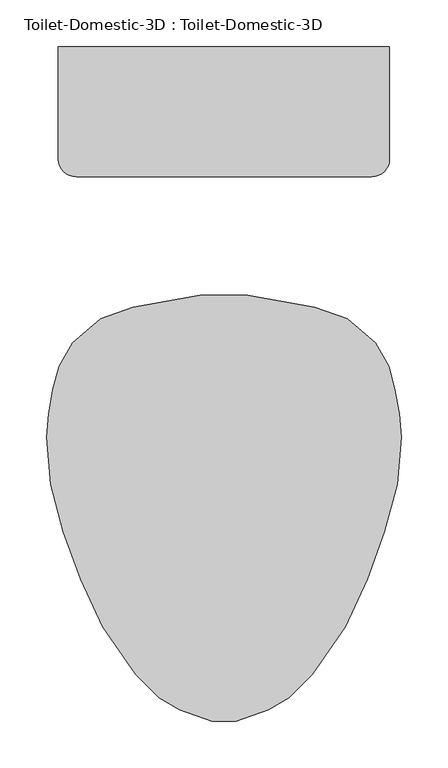
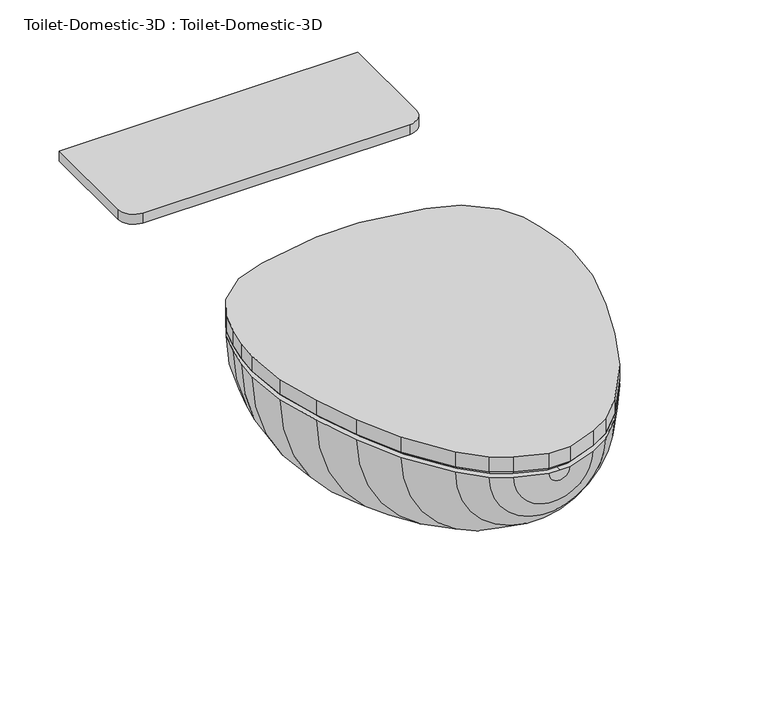
"""IFC4 building model written with IfcOpenShell, lengths in millimetres: flow terminal geometry, Toilet-Domestic-3D : Toilet-Domestic-3D."""

from ifc_helpers import new_model, si_unit, point, frame, frame_2d, origin, place, context, project, spatial, polyline, circle_curve, trimmed, segment, composite_curve, outline, extrude, faceted_brep, source, transform, mapped, element, save
from ifc_brep_helpers import plane_surface, revolved_surface, advanced_brep


def toilet_domestic_3d_toilet_domestic_3d_183bbd19(model_context):
    return source(origin(), model_context, "Body", "SolidModel", [
        advanced_brep(
        [(-25.4, 152.4, 361.95), (-97.4252791, 139.7, 361.95), (-132.3182423, 127.0, 361.95), (-162.5887836, 101.6, 361.95), (-176.9845865, 76.2, 361.95), (-183.790496, 50.8, 361.95), (-188.2862441, 25.3033453, 361.95), (-190.5, 0.0, 361.95), (-186.0724883, -50.6066907, 361.95), (-172.4088722, -101.6, 361.95), (-153.9191843, -152.4, 361.95), (-130.2307553, -203.2, 361.95), (-94.9900085, -254.0, 361.95), (-69.5900085, -279.4, 361.95), (-47.5929632, -292.1, 361.95), (-12.7, -304.8, 361.95), (0.0, -304.8, 361.95), (0.0, -284.592034, 361.95), (-12.5224565, -284.592034, 361.95), (-39.5113323, -274.7688865, 361.95), (-58.4178985, -263.8531754, 361.95), (-79.2146703, -243.0564036, 361.95), (-114.0255101, -192.8761202, 361.95), (-136.654021, -144.3491221, 361.95), (-154.575847, -95.1093097, 361.95), (-167.7238545, -46.0402777, 361.95), (-171.5645445, -2.1409906, 361.95), (-169.3087351, 23.6430284, 361.95), (-165.101298, 47.5045901, 361.95), (-159.5484355, 68.2281551, 361.95), (-146.1085923, 90.5605136, 361.95), (-121.9980886, 110.7916284, 361.95), (-94.1172813, 120.9394123, 361.95), (-22.0920022, 133.6394123, 361.95), (0.0, 133.6394123, 361.95), (0.0, 152.4, 361.95), (25.4, 152.4, 361.95), (22.0920022, 133.6394123, 361.95), (94.1172813, 120.9394123, 361.95), (121.9980886, 110.7916284, 361.95), (146.1085923, 90.5605136, 361.95), (159.5484355, 68.2281551, 361.95), (165.101298, 47.5045901, 361.95), (169.3087351, 23.6430284, 361.95), (171.5645445, -2.1409906, 361.95), (167.7238545, -46.0402777, 361.95), (154.575847, -95.1093097, 361.95), (136.654021, -144.3491221, 361.95), (114.0255101, -192.8761202, 361.95), (79.2146703, -243.0564036, 361.95), (58.4178985, -263.8531754, 361.95), (39.5113323, -274.7688865, 361.95), (12.5224565, -284.592034, 361.95), (12.7, -304.8, 361.95), (47.5929632, -292.1, 361.95), (69.5900085, -279.4, 361.95), (94.9900085, -254.0, 361.95), (130.2307553, -203.2, 361.95), (153.9191843, -152.4, 361.95), (172.4088722, -101.6, 361.95), (186.0724883, -50.6066907, 361.95), (190.5, 0.0, 361.95), (188.2862441, 25.3033453, 361.95), (183.790496, 50.8, 361.95), (176.9845865, 76.2, 361.95), (162.5887836, 101.6, 361.95), (132.3182423, 127.0, 361.95), (97.4252791, 139.7, 361.95)],
        [
            (0, 1),
            (1, 2),
            (2, 3),
            (3, 4),
            (4, 5),
            (5, 6),
            (6, 7),
            (7, 8),
            (8, 9),
            (9, 10),
            (10, 11),
            (11, 12),
            (12, 13),
            (13, 14),
            (14, 15),
            (15, 16),
            (16, 17),
            (17, 18),
            (18, 19),
            (19, 20),
            (20, 21),
            (21, 22),
            (22, 23),
            (23, 24),
            (24, 25),
            (25, 26),
            (26, 27),
            (27, 28),
            (28, 29),
            (29, 30),
            (30, 31),
            (31, 32),
            (32, 33),
            (33, 34),
            (34, 35),
            (35, 0),
            (36, 35),
            (34, 37),
            (37, 38),
            (38, 39),
            (39, 40),
            (40, 41),
            (41, 42),
            (42, 43),
            (43, 44),
            (44, 45),
            (45, 46),
            (46, 47),
            (47, 48),
            (48, 49),
            (49, 50),
            (50, 51),
            (51, 52),
            (52, 17),
            (16, 53),
            (53, 54),
            (54, 55),
            (55, 56),
            (56, 57),
            (57, 58),
            (58, 59),
            (59, 60),
            (60, 61),
            (61, 62),
            (62, 63),
            (63, 64),
            (64, 65),
            (65, 66),
            (66, 67),
            (67, 36),
            (67, 1, circle_curve(frame((0.0, 139.7, 361.95), z_axis=(0.0, 1.0, 0.0), x_axis=(-1.0, 0.0, 0.0)), 97.4252791)),
            (0, 36, circle_curve(frame((0.0, 152.4, 361.95), z_axis=(0.0, -1.0, 0.0), x_axis=(-1.0, 0.0, 0.0)), 25.4)),
            (66, 2, circle_curve(frame((0.0, 127.0, 361.95), z_axis=(0.0, 1.0, 0.0), x_axis=(-1.0, 0.0, 0.0)), 132.3182423)),
            (65, 3, circle_curve(frame((0.0, 101.6, 361.95), z_axis=(0.0, 1.0, 0.0), x_axis=(-1.0, 0.0, 0.0)), 162.5887836)),
            (64, 4, circle_curve(frame((0.0, 76.2, 361.95), z_axis=(0.0, 1.0, 0.0), x_axis=(-1.0, 0.0, 0.0)), 176.9845865)),
            (63, 5, circle_curve(frame((0.0, 50.8, 361.95), z_axis=(0.0, 1.0, 0.0), x_axis=(-1.0, 0.0, 0.0)), 183.790496)),
            (62, 6, circle_curve(frame((0.0, 25.3033453, 361.95), z_axis=(0.0, 1.0, 0.0), x_axis=(-1.0, 0.0, 0.0)), 188.2862441)),
            (61, 7, circle_curve(frame((0.0, 0.0, 361.95), z_axis=(0.0, 1.0, 0.0), x_axis=(-1.0, 0.0, 0.0)), 190.5)),
            (60, 8, circle_curve(frame((0.0, -50.6066907, 361.95), z_axis=(0.0, 1.0, 0.0), x_axis=(-1.0, 0.0, 0.0)), 186.0724883)),
            (59, 9, circle_curve(frame((0.0, -101.6, 361.95), z_axis=(0.0, 1.0, 0.0), x_axis=(-1.0, 0.0, 0.0)), 172.4088722)),
            (58, 10, circle_curve(frame((0.0, -152.4, 361.95), z_axis=(0.0, 1.0, 0.0), x_axis=(-1.0, 0.0, 0.0)), 153.9191843)),
            (57, 11, circle_curve(frame((0.0, -203.2, 361.95), z_axis=(0.0, 1.0, 0.0), x_axis=(-1.0, 0.0, 0.0)), 130.2307553)),
            (56, 12, circle_curve(frame((0.0, -254.0, 361.95), z_axis=(0.0, 1.0, 0.0), x_axis=(-1.0, 0.0, 0.0)), 94.9900085)),
            (55, 13, circle_curve(frame((0.0, -279.4, 361.95), z_axis=(0.0, 1.0, 0.0), x_axis=(-1.0, 0.0, 0.0)), 69.5900085)),
            (54, 14, circle_curve(frame((0.0, -292.1, 361.95), z_axis=(0.0, 1.0, 0.0), x_axis=(-1.0, 0.0, 0.0)), 47.5929632)),
            (53, 15, circle_curve(frame((0.0, -304.8, 361.95), z_axis=(0.0, 1.0, 0.0), x_axis=(-1.0, 0.0, 0.0)), 12.7)),
            (52, 18, circle_curve(frame((0.0, -284.592034, 361.95), z_axis=(0.0, 1.0, 0.0), x_axis=(-1.0, 0.0, 0.0)), 12.5224565)),
            (51, 19, circle_curve(frame((0.0, -274.7688865, 361.95), z_axis=(0.0, 1.0, 0.0), x_axis=(-1.0, 0.0, 0.0)), 39.5113323)),
            (50, 20, circle_curve(frame((0.0, -263.8531754, 361.95), z_axis=(0.0, 1.0, 0.0), x_axis=(-1.0, 0.0, 0.0)), 58.4178985)),
            (49, 21, circle_curve(frame((0.0, -243.0564036, 361.95), z_axis=(0.0, 1.0, 0.0), x_axis=(-1.0, 0.0, 0.0)), 79.2146703)),
            (48, 22, circle_curve(frame((0.0, -192.8761202, 361.95), z_axis=(0.0, 1.0, 0.0), x_axis=(-1.0, 0.0, 0.0)), 114.0255101)),
            (47, 23, circle_curve(frame((0.0, -144.3491221, 361.95), z_axis=(0.0, 1.0, 0.0), x_axis=(-1.0, 0.0, 0.0)), 136.654021)),
            (46, 24, circle_curve(frame((0.0, -95.1093097, 361.95), z_axis=(0.0, 1.0, 0.0), x_axis=(-1.0, 0.0, 0.0)), 154.575847)),
            (45, 25, circle_curve(frame((0.0, -46.0402777, 361.95), z_axis=(0.0, 1.0, 0.0), x_axis=(-1.0, 0.0, 0.0)), 167.7238545)),
            (44, 26, circle_curve(frame((0.0, -2.1409906, 361.95), z_axis=(0.0, 1.0, 0.0), x_axis=(-1.0, 0.0, 0.0)), 171.5645445)),
            (43, 27, circle_curve(frame((0.0, 23.6430284, 361.95), z_axis=(0.0, 1.0, 0.0), x_axis=(-1.0, 0.0, 0.0)), 169.3087351)),
            (42, 28, circle_curve(frame((0.0, 47.5045901, 361.95), z_axis=(0.0, 1.0, 0.0), x_axis=(-1.0, 0.0, 0.0)), 165.101298)),
            (41, 29, circle_curve(frame((0.0, 68.2281551, 361.95), z_axis=(0.0, 1.0, 0.0), x_axis=(-1.0, 0.0, 0.0)), 159.5484355)),
            (40, 30, circle_curve(frame((0.0, 90.5605136, 361.95), z_axis=(0.0, 1.0, 0.0), x_axis=(-1.0, 0.0, 0.0)), 146.1085923)),
            (39, 31, circle_curve(frame((0.0, 110.7916284, 361.95), z_axis=(0.0, 1.0, 0.0), x_axis=(-1.0, 0.0, 0.0)), 121.9980886)),
            (38, 32, circle_curve(frame((0.0, 120.9394123, 361.95), z_axis=(0.0, 1.0, 0.0), x_axis=(-1.0, 0.0, 0.0)), 94.1172813)),
            (37, 33, circle_curve(frame((0.0, 133.6394123, 361.95), z_axis=(0.0, 1.0, 0.0), x_axis=(-1.0, 0.0, 0.0)), 22.0920022)),
        ],
        [
            plane_surface(frame((0.0, 175.1599017, 361.95), z_axis=(0.0, 0.0, 1.0), x_axis=(-1.0, 0.0, 0.0))),
            plane_surface(frame((0.0, 175.1599017, 361.95), z_axis=(0.0, 0.0, 1.0), x_axis=(1.0, 0.0, 0.0))),
            revolved_surface(polyline([(-25.4, 152.4, 361.95), (-97.4252791, 139.7, 361.95)]), (0.0, 175.1599017, 361.95), (0.0, -1.0, 0.0)),
            revolved_surface(polyline([(-97.4252791, 139.7, 361.95), (-132.3182423, 127.0, 361.95)]), (0.0, 175.1599017, 361.95), (0.0, -1.0, 0.0)),
            revolved_surface(polyline([(-132.3182423, 127.0, 361.95), (-162.5887836, 101.6, 361.95)]), (0.0, 175.1599017, 361.95), (0.0, -1.0, 0.0)),
            revolved_surface(polyline([(-162.5887836, 101.6, 361.95), (-176.9845865, 76.2, 361.95)]), (0.0, 175.1599017, 361.95), (0.0, -1.0, 0.0)),
            revolved_surface(polyline([(-176.9845865, 76.2, 361.95), (-183.790496, 50.8, 361.95)]), (0.0, 175.1599017, 361.95), (0.0, -1.0, 0.0)),
            revolved_surface(polyline([(-183.790496, 50.8, 361.95), (-188.2862441, 25.3033453, 361.95)]), (0.0, 175.1599017, 361.95), (0.0, -1.0, 0.0)),
            revolved_surface(polyline([(-188.2862441, 25.3033453, 361.95), (-190.5, 0.0, 361.95)]), (0.0, 175.1599017, 361.95), (0.0, -1.0, 0.0)),
            revolved_surface(polyline([(-190.5, 0.0, 361.95), (-186.0724883, -50.6066907, 361.95)]), (0.0, 175.1599017, 361.95), (0.0, -1.0, 0.0)),
            revolved_surface(polyline([(-186.0724883, -50.6066907, 361.95), (-172.4088722, -101.6, 361.95)]), (0.0, 175.1599017, 361.95), (0.0, -1.0, 0.0)),
            revolved_surface(polyline([(-172.4088722, -101.6, 361.95), (-153.9191843, -152.4, 361.95)]), (0.0, 175.1599017, 361.95), (0.0, -1.0, 0.0)),
            revolved_surface(polyline([(-153.9191843, -152.4, 361.95), (-130.2307553, -203.2, 361.95)]), (0.0, 175.1599017, 361.95), (0.0, -1.0, 0.0)),
            revolved_surface(polyline([(-130.2307553, -203.2, 361.95), (-94.9900085, -254.0, 361.95)]), (0.0, 175.1599017, 361.95), (0.0, -1.0, 0.0)),
            revolved_surface(polyline([(-94.9900085, -254.0, 361.95), (-69.5900085, -279.4, 361.95)]), (0.0, 175.1599017, 361.95), (0.0, -1.0, 0.0)),
            revolved_surface(polyline([(-69.5900085, -279.4, 361.95), (-47.5929632, -292.1, 361.95)]), (0.0, 175.1599017, 361.95), (0.0, -1.0, 0.0)),
            revolved_surface(polyline([(-47.5929632, -292.1, 361.95), (-12.7, -304.8, 361.95)]), (0.0, 175.1599017, 361.95), (0.0, -1.0, 0.0)),
            plane_surface(frame((0.0, -304.8, 361.95), z_axis=(0.0, -1.0, 0.0), x_axis=(-1.0, 0.0, 0.0))),
            plane_surface(frame((0.0, -284.592034, 361.95), z_axis=(0.0, 1.0, 0.0), x_axis=(-1.0, 0.0, 0.0))),
            revolved_surface(polyline([(-12.5224565, -284.592034, 361.95), (-39.5113323, -274.7688865, 361.95)]), (0.0, 175.1599017, 361.95), (0.0, -1.0, 0.0)),
            revolved_surface(polyline([(-39.5113323, -274.7688865, 361.95), (-58.4178985, -263.8531754, 361.95)]), (0.0, 175.1599017, 361.95), (0.0, -1.0, 0.0)),
            revolved_surface(polyline([(-58.4178985, -263.8531754, 361.95), (-79.2146703, -243.0564036, 361.95)]), (0.0, 175.1599017, 361.95), (0.0, -1.0, 0.0)),
            revolved_surface(polyline([(-79.2146703, -243.0564036, 361.95), (-114.0255101, -192.8761202, 361.95)]), (0.0, 175.1599017, 361.95), (0.0, -1.0, 0.0)),
            revolved_surface(polyline([(-114.0255101, -192.8761202, 361.95), (-136.654021, -144.3491221, 361.95)]), (0.0, 175.1599017, 361.95), (0.0, -1.0, 0.0)),
            revolved_surface(polyline([(-136.654021, -144.3491221, 361.95), (-154.575847, -95.1093097, 361.95)]), (0.0, 175.1599017, 361.95), (0.0, -1.0, 0.0)),
            revolved_surface(polyline([(-154.575847, -95.1093097, 361.95), (-167.7238545, -46.0402777, 361.95)]), (0.0, 175.1599017, 361.95), (0.0, -1.0, 0.0)),
            revolved_surface(polyline([(-167.7238545, -46.0402777, 361.95), (-171.5645445, -2.1409906, 361.95)]), (0.0, 175.1599017, 361.95), (0.0, -1.0, 0.0)),
            revolved_surface(polyline([(-171.5645445, -2.1409906, 361.95), (-169.3087351, 23.6430284, 361.95)]), (0.0, 175.1599017, 361.95), (0.0, -1.0, 0.0)),
            revolved_surface(polyline([(-169.3087351, 23.6430284, 361.95), (-165.101298, 47.5045901, 361.95)]), (0.0, 175.1599017, 361.95), (0.0, -1.0, 0.0)),
            revolved_surface(polyline([(-165.101298, 47.5045901, 361.95), (-159.5484355, 68.2281551, 361.95)]), (0.0, 175.1599017, 361.95), (0.0, -1.0, 0.0)),
            revolved_surface(polyline([(-159.5484355, 68.2281551, 361.95), (-146.1085923, 90.5605136, 361.95)]), (0.0, 175.1599017, 361.95), (0.0, -1.0, 0.0)),
            revolved_surface(polyline([(-146.1085923, 90.5605136, 361.95), (-121.9980886, 110.7916284, 361.95)]), (0.0, 175.1599017, 361.95), (0.0, -1.0, 0.0)),
            revolved_surface(polyline([(-121.9980886, 110.7916284, 361.95), (-94.1172813, 120.9394123, 361.95)]), (0.0, 175.1599017, 361.95), (0.0, -1.0, 0.0)),
            revolved_surface(polyline([(-94.1172813, 120.9394123, 361.95), (-22.0920022, 133.6394123, 361.95)]), (0.0, 175.1599017, 361.95), (0.0, -1.0, 0.0)),
            plane_surface(frame((0.0, 133.6394123, 361.95), z_axis=(0.0, -1.0, 0.0), x_axis=(-1.0, 0.0, 0.0))),
            plane_surface(frame((0.0, 152.4, 361.95), z_axis=(0.0, 1.0, 0.0), x_axis=(-1.0, 0.0, 0.0))),
        ],
        [
            (0, [[1, 2, 3, 4, 5, 6, 7, 8, 9, 10, 11, 12, 13, 14, 15, 16, 17, 18, 19, 20, 21, 22, 23, 24, 25, 26, 27, 28, 29, 30, 31, 32, 33, 34, 35, 36]]),
            (1, [[37, -35, 38, 39, 40, 41, 42, 43, 44, 45, 46, 47, 48, 49, 50, 51, 52, 53, 54, -17, 55, 56, 57, 58, 59, 60, 61, 62, 63, 64, 65, 66, 67, 68, 69, 70]]),
            (2, [[71, -1, 72, -70]]),
            (3, [[73, -2, -71, -69]]),
            (4, [[74, -3, -73, -68]]),
            (5, [[75, -4, -74, -67]]),
            (6, [[76, -5, -75, -66]]),
            (7, [[77, -6, -76, -65]]),
            (8, [[78, -7, -77, -64]]),
            (9, [[79, -8, -78, -63]]),
            (10, [[80, -9, -79, -62]]),
            (11, [[81, -10, -80, -61]]),
            (12, [[82, -11, -81, -60]]),
            (13, [[83, -12, -82, -59]]),
            (14, [[84, -13, -83, -58]]),
            (15, [[85, -14, -84, -57]]),
            (16, [[86, -15, -85, -56]]),
            (17, [[-16, -86, -55]]),
            (18, [[87, -18, -54]]),
            (19, [[88, -19, -87, -53]]),
            (20, [[89, -20, -88, -52]]),
            (21, [[90, -21, -89, -51]]),
            (22, [[91, -22, -90, -50]]),
            (23, [[92, -23, -91, -49]]),
            (24, [[93, -24, -92, -48]]),
            (25, [[94, -25, -93, -47]]),
            (26, [[95, -26, -94, -46]]),
            (27, [[96, -27, -95, -45]]),
            (28, [[97, -28, -96, -44]]),
            (29, [[98, -29, -97, -43]]),
            (30, [[99, -30, -98, -42]]),
            (31, [[100, -31, -99, -41]]),
            (32, [[101, -32, -100, -40]]),
            (33, [[102, -33, -101, -39]]),
            (34, [[-34, -102, -38]]),
            (35, [[-72, -36, -37]]),
        ],
    ),
        faceted_brep([(-97.4252791, 139.7, 368.3), (-132.3182423, 127.0, 368.3), (-162.5887836, 101.6, 368.3), (-176.9845865, 76.2, 368.3), (-183.790496, 50.8, 368.3), (-188.2862441, 25.3033453, 368.3), (-190.5, 0.0, 368.3), (-186.0724883, -50.6066907, 368.3), (-172.4088722, -101.6, 368.3), (-153.9191843, -152.4, 368.3), (-130.2307553, -203.2, 368.3), (-94.9900085, -254.0, 368.3), (-69.5900085, -279.4, 368.3), (-47.5929632, -292.1, 368.3), (-12.7, -304.8, 368.3), (12.7, -304.8, 368.3), (47.5929632, -292.1, 368.3), (69.5900085, -279.4, 368.3), (94.9900085, -254.0, 368.3), (130.2307553, -203.2, 368.3), (153.9191843, -152.4, 368.3), (172.4088722, -101.6, 368.3), (186.0724883, -50.6066907, 368.3), (190.5, 0.0, 368.3), (188.2862441, 25.3033453, 368.3), (183.790496, 50.8, 368.3), (176.9845865, 76.2, 368.3), (162.5887836, 101.6, 368.3), (132.3182423, 127.0, 368.3), (97.4252791, 139.7, 368.3), (25.4, 152.4, 368.3), (-25.4, 152.4, 368.3), (-95.7755003, 133.5429415, 361.95), (-24.844447, 146.05, 361.95), (24.844447, 146.05, 361.95), (95.7755003, 133.5429415, 361.95), (129.0942628, 121.4159037, 361.95), (157.6293435, 97.472128, 361.95), (171.060664, 73.773864, 361.95), (177.5851102, 49.4242991, 361.95), (181.9845715, 24.4737144, 361.95), (184.125744, 0.0, 361.95), (179.7950716, -49.4998127, 361.95), (166.347, -99.688699, 361.95), (148.0469602, -149.9676451, 361.95), (124.7045808, -200.0255393, 361.95), (90.0971582, -249.9125941, 361.95), (65.691017, -274.3187354, 361.95), (44.8990862, -286.3229622, 361.95), (11.5803237, -298.45, 361.95), (-11.5803237, -298.45, 361.95), (-44.8990862, -286.3229622, 361.95), (-65.691017, -274.3187354, 361.95), (-90.0971582, -249.9125941, 361.95), (-124.7045808, -200.0255393, 361.95), (-148.0469602, -149.9676451, 361.95), (-166.347, -99.688699, 361.95), (-179.7950716, -49.4998127, 361.95), (-184.125744, 0.0, 361.95), (-181.9845715, 24.4737144, 361.95), (-177.5851102, 49.4242991, 361.95), (-171.060664, 73.773864, 361.95), (-157.6293435, 97.472128, 361.95), (-129.0942628, 121.4159037, 361.95)], [[[0, 1, 2, 3, 4, 5, 6, 7, 8, 9, 10, 11, 12, 13, 14, 15, 16, 17, 18, 19, 20, 21, 22, 23, 24, 25, 26, 27, 28, 29, 30, 31]], [[32, 33, 34, 35, 36, 37, 38, 39, 40, 41, 42, 43, 44, 45, 46, 47, 48, 49, 50, 51, 52, 53, 54, 55, 56, 57, 58, 59, 60, 61, 62, 63]], [[32, 63, 1, 0]], [[63, 62, 2, 1]], [[62, 61, 3, 2]], [[61, 60, 4, 3]], [[60, 59, 5, 4]], [[59, 58, 6, 5]], [[58, 57, 7, 6]], [[57, 56, 8, 7]], [[56, 55, 9, 8]], [[55, 54, 10, 9]], [[54, 53, 11, 10]], [[53, 52, 12, 11]], [[52, 51, 13, 12]], [[51, 50, 14, 13]], [[50, 49, 15, 14]], [[49, 48, 16, 15]], [[48, 47, 17, 16]], [[47, 46, 18, 17]], [[46, 45, 19, 18]], [[45, 44, 20, 19]], [[44, 43, 21, 20]], [[43, 42, 22, 21]], [[42, 41, 23, 22]], [[41, 40, 24, 23]], [[40, 39, 25, 24]], [[39, 38, 26, 25]], [[38, 37, 27, 26]], [[37, 36, 28, 27]], [[36, 35, 29, 28]], [[35, 34, 30, 29]], [[34, 33, 31, 30]], [[33, 32, 0, 31]]]),
        extrude(outline(composite_curve([segment(polyline([(177.8, 419.1), (177.8, 298.45)]), True, "CONTINUOUS"), segment(trimmed(circle_curve(frame_2d((158.75, 298.45)), 19.05), [point((177.8, 298.45))], [point((158.75, 279.4))], False, "CARTESIAN"), True, "CONTINUOUS"), segment(polyline([(158.75, 279.4), (-158.75, 279.4)]), True, "CONTINUOUS"), segment(trimmed(circle_curve(frame_2d((-158.75, 298.45)), 19.05), [point((-158.75, 279.4))], [point((-177.8, 298.45))], False, "CARTESIAN"), True, "CONTINUOUS"), segment(polyline([(-177.8, 298.45), (-177.8, 419.1), (177.8, 419.1)]), True, "CONTINUOUS")], self_intersect=False)), frame((0.0, 0.0, 374.65), z_axis=(0.0, 0.0, 1.0), x_axis=(1.0, 0.0, 0.0)), (0.0, 0.0, 1.0), 12.5681453),
        extrude(outline(polyline([(-162.5887836, 101.6), (-132.3182423, 127.0), (-97.4252791, 139.7), (-25.4, 152.4), (25.4, 152.4), (97.4252791, 139.7), (132.3182423, 127.0), (162.5887836, 101.6), (176.9845865, 76.2), (183.790496, 50.8), (188.2862441, 25.3033453), (190.5, 0.0), (186.0724883, -50.6066907), (172.4088722, -101.6), (153.9191843, -152.4), (130.2307553, -203.2), (94.9900085, -254.0), (69.5900085, -279.4), (47.5929632, -292.1), (12.7, -304.8), (-12.7, -304.8), (-47.5929632, -292.1), (-69.5900085, -279.4), (-94.9900085, -254.0), (-130.2307553, -203.2), (-153.9191843, -152.4), (-172.4088722, -101.6), (-186.0724883, -50.6066907), (-190.5, 0.0), (-188.2862441, 25.3033453), (-183.790496, 50.8), (-176.9845865, 76.2), (-162.5887836, 101.6)])), frame((0.0, 0.0, 368.3), z_axis=(0.0, 0.0, 1.0), x_axis=(1.0, 0.0, 0.0)), (0.0, 0.0, 1.0), 19.05),
    ])


if __name__ == "__main__":
    model = new_model("IFC4")
    model_context = context("Model", 3, world=origin())
    ifc_project = project(units=[si_unit("LENGTHUNIT", "METRE", prefix="MILLI")], contexts=[model_context])
    site = spatial("IfcSite", under=ifc_project)
    building = spatial("IfcBuilding", under=site)
    placement = place(None, origin())
    toilet_domestic_3d_toilet_domestic_3d_shape = toilet_domestic_3d_toilet_domestic_3d_183bbd19(model_context)
    element("IfcFlowTerminal", 1, ObjectType="Toilet-Domestic-3D : Toilet-Domestic-3D", at=placement, inside=building, context=model_context, shape_type="MappedRepresentation", body=[
        mapped(toilet_domestic_3d_toilet_domestic_3d_shape, transform((0.0, 0.0, 0.0), x_axis=(1.0, 0.0, 0.0), y_axis=(0.0, 1.0, 0.0), z_axis=(0.0, 0.0, 1.0))),
    ])
    save(model, "model.ifc")

# Revit data of these elements
# Type "Toilet-Domestic-3D : Toilet-Domestic-3D"
#   Assembly Code = "D2010110"
#   Toilet - Bowl/Basin Material = Porcelain, Linen
#   Toilet - Seat Material = Laminate, Linen, Matte
#   Default Elevation = 0
# Element 1 (IfcFlowTerminal, "Toilet-Domestic-3D : Toilet-Domestic-3D")
#   Materials on its faces: "Porcelain, Linen", "Laminate, Linen, Matte"
# Materials
#   "Porcelain, Linen": class "Ceramic", colour RGB 249 239 230, transparency 0, Description = "Porcelain, linen", Cost = 0
#   "Laminate, Linen, Matte": class "Plastic", colour RGB 249 239 230, transparency 0, Description = "Plastic Laminate - Linen, Matte", Cost = 0
